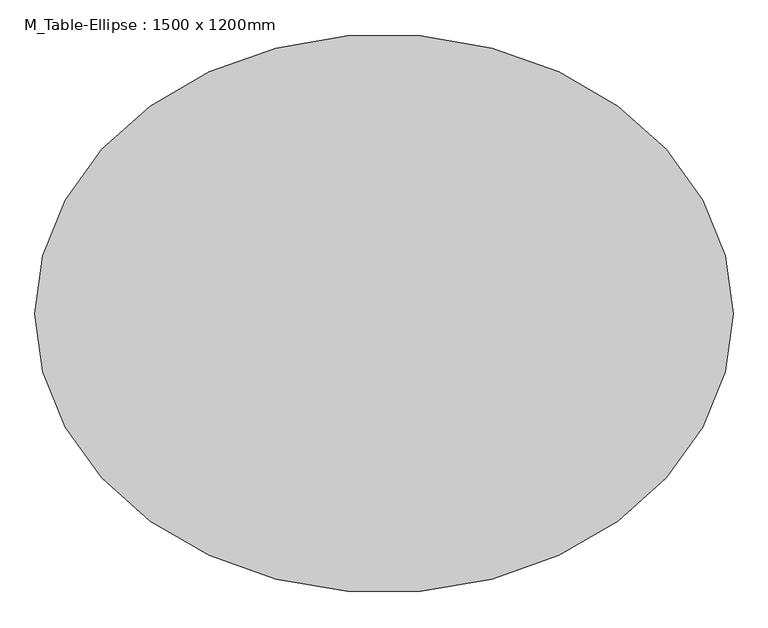
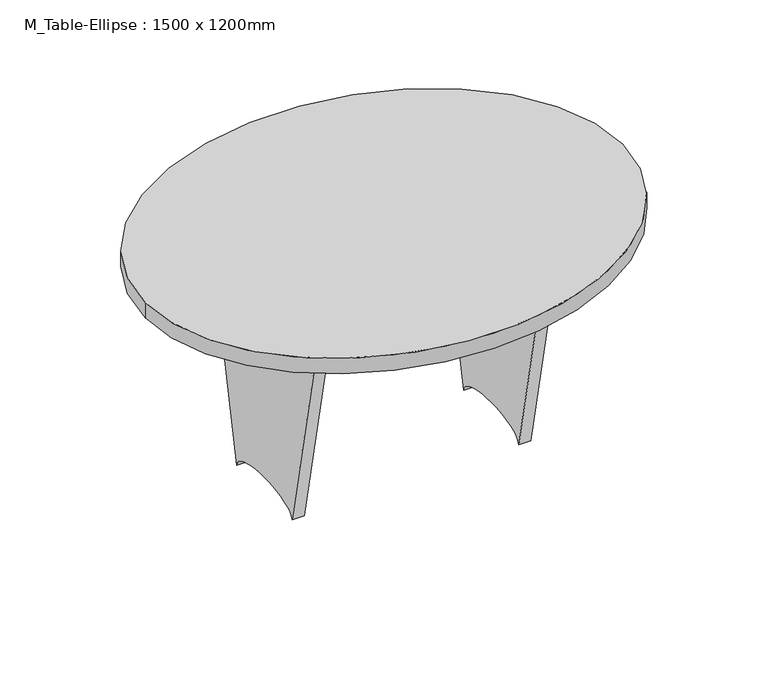
"""IFC4 building model written with IfcOpenShell, lengths in millimetres: furniture geometry, M_Table-Ellipse : 1500 x 1200mm."""

from ifc_helpers import new_model, si_unit, point, frame, origin, place, context, project, spatial, ellipse_curve, trimmed, source, transform, mapped, element, save
from ifc_brep_helpers import plane_surface, extruded_surface, advanced_brep


def m_table_ellipse_1500_x_1200mm_3917c766(model_context):
    return source(origin(), model_context, "Body", "AdvancedBrep", [
        advanced_brep(
        [(-336.9, 19.05, 711.2), (336.9, 19.05, 711.2), (336.9, 19.05, 474.1333333), (-336.9, 19.05, 474.1333333), (-336.9, -19.05, 711.2), (-336.9, -19.05, 474.1333333), (336.9, -19.05, 474.1333333), (336.9, -19.05, 711.2)],
        [
            (0, 1),
            (1, 2),
            (2, 3, ellipse_curve(frame((0.0, 19.05, 474.1333333), z_axis=(0.0, -1.0, 0.0), x_axis=(1.0, 0.0, 0.0)), 336.9, 101.6)),
            (3, 0),
            (4, 5),
            (5, 6, ellipse_curve(frame((0.0, -19.05, 474.1333333), z_axis=(0.0, 1.0, 0.0), x_axis=(1.0, 0.0, 0.0)), 336.9, 101.6)),
            (6, 7),
            (7, 4),
            (0, 4),
            (7, 1),
            (6, 2),
            (5, 3),
        ],
        [
            plane_surface(frame((-336.9, 19.05, 711.2), z_axis=(0.0, 1.0, 0.0), x_axis=(1.0, 0.0, 0.0))),
            plane_surface(frame((-336.9, -19.05, 711.2), z_axis=(0.0, -1.0, 0.0), x_axis=(-1.0, 0.0, 0.0))),
            plane_surface(frame((-336.9, 19.05, 711.2), z_axis=(0.0, 0.0, 1.0), x_axis=(0.0, -1.0, 0.0))),
            plane_surface(frame((336.9, 19.05, 711.2), z_axis=(1.0, 0.0, 0.0), x_axis=(0.0, -1.0, 0.0))),
            extruded_surface(trimmed(ellipse_curve(frame((0.0, -57.15, 474.1333333), z_axis=(0.0, -1.0, 0.0), x_axis=(1.0, 0.0, 0.0)), 336.9, 101.6), [point((336.9, -57.15, 474.1333333))], [point((-336.9, -57.15, 474.1333333))], True, "CARTESIAN"), (0.0, 38.099999999999994, 0.0), 38.099999999999994),
            plane_surface(frame((-336.9, 19.05, 474.1333333), z_axis=(-1.0, 0.0, 0.0), x_axis=(0.0, -1.0, 0.0))),
        ],
        [
            (0, [[1, 2, 3, 4]]),
            (1, [[5, 6, 7, 8]]),
            (2, [[-1, 9, -8, 10]]),
            (3, [[-2, -10, -7, 11]]),
            (4, [[-3, -11, -6, 12]]),
            (5, [[-4, -12, -5, -9]]),
        ],
    ),
        advanced_brep(
        [(375.0, 300.0, 711.2), (375.0, -300.0, 711.2), (375.0, -150.0, 0.0), (375.0, 150.0, 0.0), (336.9, 300.0, 711.2), (336.9, 150.0, 0.0), (336.9, -150.0, 0.0), (336.9, -300.0, 711.2)],
        [
            (0, 1),
            (1, 2),
            (2, 3, ellipse_curve(frame((375.0, 0.0, 0.0), z_axis=(-1.0, 0.0, 0.0), x_axis=(0.0, 1.0, 0.0)), 150.0, 50.8)),
            (3, 0),
            (4, 5),
            (5, 6, ellipse_curve(frame((336.9, 0.0, 0.0), z_axis=(1.0, 0.0, 0.0), x_axis=(0.0, 1.0, 0.0)), 150.0, 50.8)),
            (6, 7),
            (7, 4),
            (0, 4),
            (7, 1),
            (6, 2),
            (5, 3),
        ],
        [
            plane_surface(frame((375.0, -300.0, 711.2), z_axis=(1.0, 0.0, 0.0), x_axis=(0.0, -1.0, 0.0))),
            plane_surface(frame((336.9, -300.0, 711.2), z_axis=(-1.0, 0.0, 0.0), x_axis=(0.0, 1.0, 0.0))),
            plane_surface(frame((375.0, 300.0, 711.2), z_axis=(0.0, 0.0, 1.0), x_axis=(-1.0, 0.0, 0.0))),
            plane_surface(frame((375.0, -300.0, 711.2), z_axis=(0.0, -0.9784738119782022, -0.20637102333623775), x_axis=(-1.0, 0.0, 0.0))),
            extruded_surface(trimmed(ellipse_curve(frame((298.8, 0.0, 0.0), z_axis=(-1.0, 0.0, 0.0), x_axis=(0.0, 1.0, 0.0)), 150.0, 50.8), [point((298.8, -150.0, 0.0))], [point((298.8, 150.0, 0.0))], True, "CARTESIAN"), (38.099999999999966, 0.0, 0.0), 38.099999999999966),
            plane_surface(frame((375.0, 150.0, 0.0), z_axis=(0.0, 0.978473811978203, -0.20637102333623358), x_axis=(-1.0, 0.0, 0.0))),
        ],
        [
            (0, [[1, 2, 3, 4]]),
            (1, [[5, 6, 7, 8]]),
            (2, [[-1, 9, -8, 10]]),
            (3, [[-2, -10, -7, 11]]),
            (4, [[-3, -11, -6, 12]]),
            (5, [[-4, -12, -5, -9]]),
        ],
    ),
        advanced_brep(
        [(-336.9, 300.0, 711.2), (-336.9, -300.0, 711.2), (-336.9, -150.0, 0.0), (-336.9, 150.0, 0.0), (-375.0, 300.0, 711.2), (-375.0, 150.0, 0.0), (-375.0, -150.0, 0.0), (-375.0, -300.0, 711.2)],
        [
            (0, 1),
            (1, 2),
            (2, 3, ellipse_curve(frame((-336.9, 0.0, 0.0), z_axis=(-1.0, 0.0, 0.0), x_axis=(0.0, 1.0, 0.0)), 150.0, 50.8)),
            (3, 0),
            (4, 5),
            (5, 6, ellipse_curve(frame((-375.0, 0.0, 0.0), z_axis=(1.0, 0.0, 0.0), x_axis=(0.0, 1.0, 0.0)), 150.0, 50.8)),
            (6, 7),
            (7, 4),
            (0, 4),
            (7, 1),
            (6, 2),
            (5, 3),
        ],
        [
            plane_surface(frame((-336.9, -300.0, 711.2), z_axis=(1.0, 0.0, 0.0), x_axis=(0.0, -1.0, 0.0))),
            plane_surface(frame((-375.0, -300.0, 711.2), z_axis=(-1.0, 0.0, 0.0), x_axis=(0.0, 1.0, 0.0))),
            plane_surface(frame((-336.9, 300.0, 711.2), z_axis=(0.0, 0.0, 1.0), x_axis=(-1.0, 0.0, 0.0))),
            plane_surface(frame((-336.9, -300.0, 711.2), z_axis=(0.0, -0.9784738119782, -0.20637102333624732), x_axis=(-1.0, 0.0, 0.0))),
            extruded_surface(trimmed(ellipse_curve(frame((-413.1, 0.0, 0.0), z_axis=(-1.0, 0.0, 0.0), x_axis=(0.0, 1.0, 0.0)), 150.0, 50.8), [point((-413.1, -150.0, 0.0))], [point((-413.1, 150.0, 0.0))], True, "CARTESIAN"), (38.10000000000002, 0.0, 0.0), 38.10000000000002),
            plane_surface(frame((-336.9, 150.0, 0.0), z_axis=(0.0, 0.9784738119782022, -0.2063710233362382), x_axis=(-1.0, 0.0, 0.0))),
        ],
        [
            (0, [[1, 2, 3, 4]]),
            (1, [[5, 6, 7, 8]]),
            (2, [[-1, 9, -8, 10]]),
            (3, [[-2, -10, -7, 11]]),
            (4, [[-3, -11, -6, 12]]),
            (5, [[-4, -12, -5, -9]]),
        ],
    ),
        advanced_brep(
        [(-750.0, 0.0, 762.0), (750.0, 0.0, 762.0), (-750.0, 0.0, 711.2), (750.0, 0.0, 711.2)],
        [
            (0, 1, ellipse_curve(frame((0.0, 0.0, 762.0), z_axis=(0.0, 0.0, 1.0), x_axis=(1.0, 0.0, 0.0)), 750.0, 600.0)),
            (1, 0, ellipse_curve(frame((0.0, 0.0, 762.0), z_axis=(0.0, 0.0, 1.0), x_axis=(1.0, 0.0, 0.0)), 750.0, 600.0)),
            (2, 3, ellipse_curve(frame((0.0, 0.0, 711.2), z_axis=(0.0, 0.0, -1.0), x_axis=(1.0, 0.0, 0.0)), 750.0, 600.0)),
            (3, 2, ellipse_curve(frame((0.0, 0.0, 711.2), z_axis=(0.0, 0.0, -1.0), x_axis=(1.0, 0.0, 0.0)), 750.0, 600.0)),
            (0, 2),
            (3, 1),
        ],
        [
            plane_surface(frame((750.0, 0.0, 762.0), z_axis=(0.0, 0.0, 1.0), x_axis=(0.0, 1.0, 0.0))),
            plane_surface(frame((750.0, 0.0, 711.2), z_axis=(0.0, 0.0, -1.0), x_axis=(0.0, -1.0, 0.0))),
            extruded_surface(trimmed(ellipse_curve(frame((0.0, 0.0, 660.4), z_axis=(0.0, 0.0, 1.0), x_axis=(1.0, 0.0, 0.0)), 750.0, 600.0), [point((-750.0, 0.0, 660.4))], [point((750.0, 0.0, 660.4))], True, "CARTESIAN"), (0.0, 0.0, 50.80000000000007), 50.80000000000007),
            extruded_surface(trimmed(ellipse_curve(frame((0.0, 0.0, 660.4), z_axis=(0.0, 0.0, 1.0), x_axis=(1.0, 0.0, 0.0)), 750.0, 600.0), [point((750.0, 0.0, 660.4))], [point((-750.0, 0.0, 660.4))], True, "CARTESIAN"), (0.0, 0.0, 50.80000000000007), 50.80000000000007),
        ],
        [
            (0, [[1, 2]]),
            (1, [[3, 4]]),
            (2, [[-1, 5, -4, 6]]),
            (3, [[-2, -6, -3, -5]]),
        ],
    ),
    ])


if __name__ == "__main__":
    model = new_model("IFC4")
    model_context = context("Model", 3, world=origin())
    ifc_project = project(units=[si_unit("LENGTHUNIT", "METRE", prefix="MILLI")], contexts=[model_context])
    site = spatial("IfcSite", under=ifc_project)
    building = spatial("IfcBuilding", under=site)
    placement = place(None, origin())
    m_table_ellipse_1500_x_1200mm_shape = m_table_ellipse_1500_x_1200mm_3917c766(model_context)
    element("IfcFurniture", 1, ObjectType="M_Table-Ellipse : 1500 x 1200mm", at=placement, inside=building, context=model_context, shape_type="MappedRepresentation", body=[
        mapped(m_table_ellipse_1500_x_1200mm_shape, transform((0.0, 0.0, 0.0), x_axis=(1.0, 0.0, 0.0), y_axis=(0.0, 1.0, 0.0), z_axis=(0.0, 0.0, 1.0))),
    ])
    save(model, "model.ifc")

# Revit data of these elements
# Type "M_Table-Ellipse : 1500 x 1200mm"
#   Half Width = 600 mm
#   Half Length = 750 mm
#   Height = 762 mm
#   Length = 1500 mm
#   Width = 1200 mm
#   Base Material = Birch
#   Top Material = Birch
#   Default Elevation = 0
#   Assembly Code = ""
# Element 1 (IfcFurniture, "M_Table-Ellipse : 1500 x 1200mm")
#   Materials on its faces: "Birch"
# Materials
#   "Birch": class "Wood", colour RGB 224 178 126, transparency 0, Description = "Betula Alleghaniensis", Cost = 0
